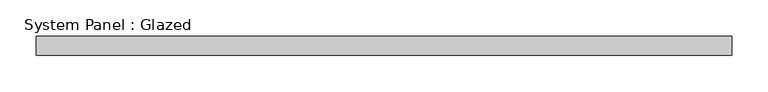
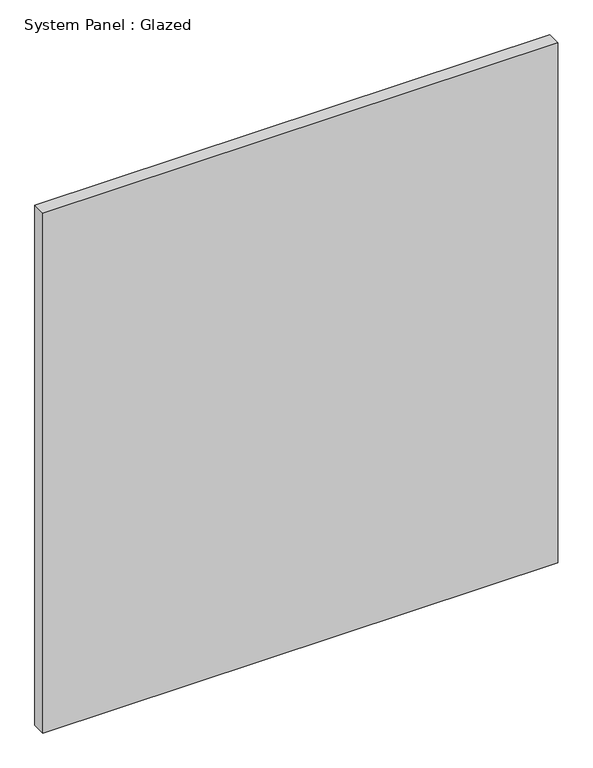
"""IFC4 building model written with IfcOpenShell, lengths in millimetres: plate geometry, System Panel : Glazed."""

from ifc_helpers import new_model, si_unit, origin, origin_with_axes, place, context, project, spatial, polyline, outline, extrude, source, transform, mapped, element, save


def system_panel_glazed_c8b910d9(model_context):
    return source(origin(), model_context, "Body", "SweptSolid", [
        extrude(outline(polyline([(476.3206338, 19.05), (-476.3206338, 19.05), (-476.3206338, 44.45), (476.3206338, 44.45), (476.3206338, 19.05)])), origin_with_axes(), (0.0, 0.0, 1.0), 1016.2501856),
    ])


if __name__ == "__main__":
    model = new_model("IFC4")
    model_context = context("Model", 3, world=origin())
    ifc_project = project(units=[si_unit("LENGTHUNIT", "METRE", prefix="MILLI")], contexts=[model_context])
    site = spatial("IfcSite", under=ifc_project)
    building = spatial("IfcBuilding", under=site)
    placement = place(None, origin())
    system_panel_glazed_shape = system_panel_glazed_c8b910d9(model_context)
    element("IfcPlate", 1, ObjectType="System Panel : Glazed", at=placement, inside=building, context=model_context, shape_type="MappedRepresentation", body=[
        mapped(system_panel_glazed_shape, transform((0.0, 0.0, 0.0), x_axis=(1.0, 0.0, 0.0), y_axis=(0.0, 1.0, 0.0), z_axis=(0.0, 0.0, 1.0))),
    ])
    save(model, "model.ifc")

# Revit data of these elements
# Type "System Panel : Glazed"
#   Construction Type Id = "GSP4R"
#   Analytic Construction = "1/8 in Pilkington single glazing"
#   Visual Light Transmittance = 0.9
#   Solar Heat Gain Coefficient = 0.86
#   Heat Transfer Coefficient (U) = 1.18115 BTU/(h·ft²·°F)
#   Define Thermal Properties by = 1
# Element 1 (IfcPlate, "System Panel : Glazed")
#   Materials on its faces: "Glass"
# Materials
#   "Glass": class "Glass", colour RGB 0 128 192, transparency 0.75, Description = "Soda Lime Glass", Cost = 0
